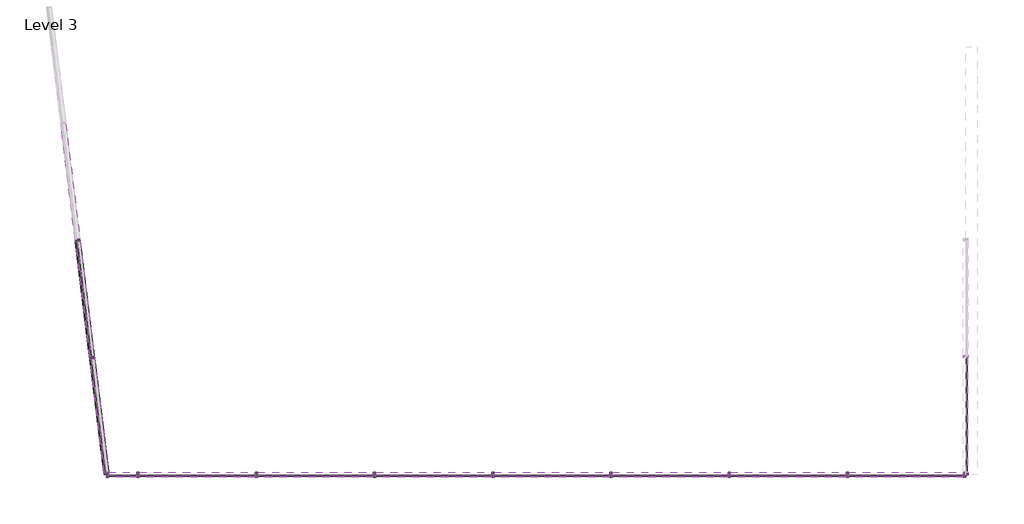
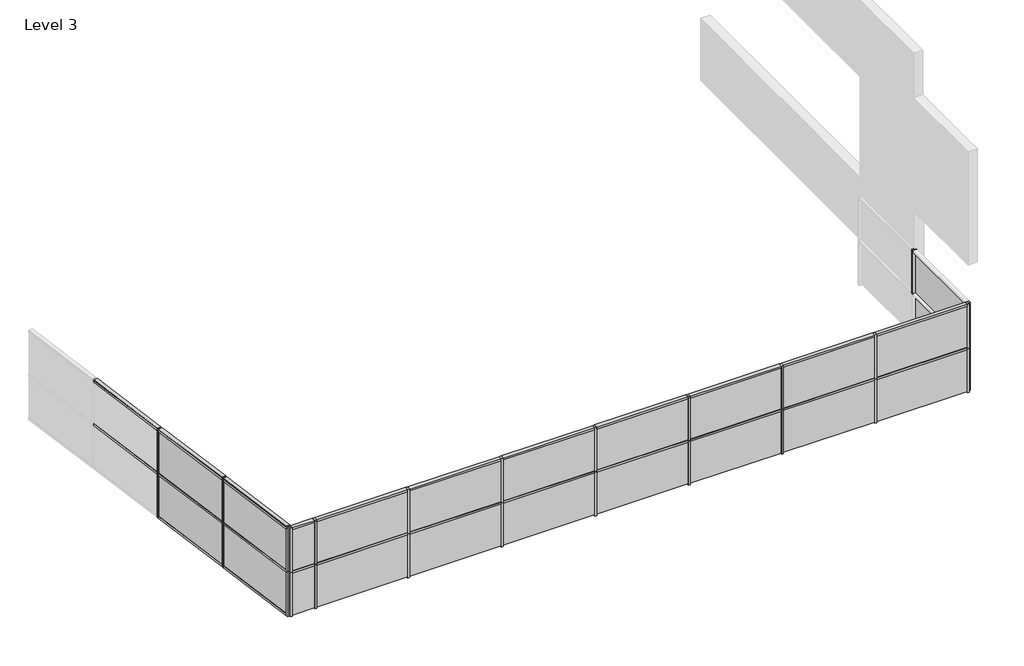
# One storey, part 1 of 2: 63 members, 26 plates.
"""IFC4 building model written with IfcOpenShell, lengths in millimetres."""

from ifc_helpers import new_model, si_unit, origin, place, context, project, spatial, transform, mapped, element, save
from components import member_71c27fd2, member_daa7a266, member_82905deb, member_19d0a4ec, member_8cef0660, member_db480205, member_4491d118, member_0c11e56c, member_695b83e4, system_panel_glazed_37f15d2e, system_panel_glazed_3620f98e, system_panel_glazed_e46d4b42, system_panel_glazed_2a6c68b7, system_panel_glazed_07b088f8, system_panel_glazed_9d0e0944

model = new_model("IFC4")

# Units and contexts
model_context = context("Model", 3, world=origin())
ifc_project = project(units=[si_unit("LENGTHUNIT", "METRE", prefix="MILLI")], contexts=[model_context])

# Site, building, storey
site = spatial("IfcSite", under=ifc_project)
building = spatial("IfcBuilding", under=site)
storey = spatial("IfcBuildingStorey", under=building, Name="Level 3", Elevation=6096.0)

# Members
placement = place(None, origin())
member_shape = member_71c27fd2(model_context)
element("IfcMember", 1, ObjectType="Rectangular Mullion : 2.5\" x 5\" rectangular", at=placement, inside=storey, context=model_context, shape_type="MappedRepresentation", body=[
    mapped(member_shape, transform((-8620.3262186, -3985.3690403, 6096.0), x_axis=(0.0, 0.0, -1.0), y_axis=(-0.9925461516413222, -0.12186934340514607, 0.0), z_axis=(-0.12186934340514607, 0.9925461516413222, 0.0))),
])
member_2_shape = member_daa7a266(model_context)
element("IfcMember", 2, ObjectType="Rectangular Mullion : 2.5\" x 5\" rectangular", at=placement, inside=storey, context=model_context, shape_type="MappedRepresentation", body=[
    mapped(member_2_shape, transform((-8260.4765148, -6916.1096898, 9144.0), x_axis=(0.0, 0.0, 1.0), y_axis=(-0.9925461516413222, -0.12186934340514603, 0.0), z_axis=(0.12186934340514603, -0.9925461516413222, 0.0))),
])
element("IfcMember", 3, ObjectType="Rectangular Mullion : 2.5\" x 5\" rectangular", at=placement, inside=storey, context=model_context, shape_type="MappedRepresentation", body=[
    mapped(member_2_shape, transform((13839.0156363, -6979.1363705, 9144.0), x_axis=(0.0, 0.0, 1.0), y_axis=(0.0, -1.0, 0.0), z_axis=(1.0, 0.0, 0.0))),
])
member_3_shape = member_82905deb(model_context)
element("IfcMember", 4, ObjectType="Rectangular Mullion : 2.5\" x 5\" rectangular", at=placement, inside=storey, context=model_context, shape_type="MappedRepresentation", body=[
    mapped(member_3_shape, transform((-8624.1955702, -3953.8557, 9144.0), x_axis=(-0.12186934340514591, 0.9925461516413222, 0.0), y_axis=(-0.9925461516413222, -0.12186934340514591, 0.0), z_axis=(0.0, 0.0, 1.0))),
])
element("IfcMember", 5, ObjectType="Rectangular Mullion : 2.5\" x 5\" rectangular", at=placement, inside=storey, context=model_context, shape_type="MappedRepresentation", body=[
    mapped(member_3_shape, transform((-8995.6533289, -928.5750297, 9144.0), x_axis=(-0.12186934340514591, 0.9925461516413222, 0.0), y_axis=(-0.9925461516413222, -0.12186934340514591, 0.0), z_axis=(0.0, 0.0, 1.0))),
])
element("IfcMember", 6, ObjectType="Rectangular Mullion : 2.5\" x 5\" rectangular", at=placement, inside=storey, context=model_context, shape_type="MappedRepresentation", body=[
    mapped(member_3_shape, transform((10854.515636, -6979.1363705, 9144.0), x_axis=(-1.0, 0.0, 0.0), y_axis=(0.0, -1.0, 0.0), z_axis=(0.0, 0.0, 1.0))),
])
element("IfcMember", 7, ObjectType="Rectangular Mullion : 2.5\" x 5\" rectangular", at=placement, inside=storey, context=model_context, shape_type="MappedRepresentation", body=[
    mapped(member_3_shape, transform((7806.515636, -6979.1363705, 9144.0), x_axis=(-1.0, 0.0, 0.0), y_axis=(0.0, -1.0, 0.0), z_axis=(0.0, 0.0, 1.0))),
])
element("IfcMember", 8, ObjectType="Rectangular Mullion : 2.5\" x 5\" rectangular", at=placement, inside=storey, context=model_context, shape_type="MappedRepresentation", body=[
    mapped(member_3_shape, transform((4758.515636, -6979.1363705, 9144.0), x_axis=(-1.0, 0.0, 0.0), y_axis=(0.0, -1.0, 0.0), z_axis=(0.0, 0.0, 1.0))),
])
element("IfcMember", 9, ObjectType="Rectangular Mullion : 2.5\" x 5\" rectangular", at=placement, inside=storey, context=model_context, shape_type="MappedRepresentation", body=[
    mapped(member_3_shape, transform((1710.515636, -6979.1363705, 9144.0), x_axis=(-1.0, 0.0, 0.0), y_axis=(0.0, -1.0, 0.0), z_axis=(0.0, 0.0, 1.0))),
])
element("IfcMember", 10, ObjectType="Rectangular Mullion : 2.5\" x 5\" rectangular", at=placement, inside=storey, context=model_context, shape_type="MappedRepresentation", body=[
    mapped(member_3_shape, transform((-1337.484364, -6979.1363705, 9144.0), x_axis=(-1.0, 0.0, 0.0), y_axis=(0.0, -1.0, 0.0), z_axis=(0.0, 0.0, 1.0))),
])
element("IfcMember", 11, ObjectType="Rectangular Mullion : 2.5\" x 5\" rectangular", at=placement, inside=storey, context=model_context, shape_type="MappedRepresentation", body=[
    mapped(member_3_shape, transform((-4385.484364, -6979.1363705, 9144.0), x_axis=(-1.0, 0.0, 0.0), y_axis=(0.0, -1.0, 0.0), z_axis=(0.0, 0.0, 1.0))),
])
element("IfcMember", 12, ObjectType="Rectangular Mullion : 2.5\" x 5\" rectangular", at=placement, inside=storey, context=model_context, shape_type="MappedRepresentation", body=[
    mapped(member_3_shape, transform((-7433.484364, -6979.1363705, 9144.0), x_axis=(-1.0, 0.0, 0.0), y_axis=(0.0, -1.0, 0.0), z_axis=(0.0, 0.0, 1.0))),
])
element("IfcMember", 13, ObjectType="Rectangular Mullion : 2.5\" x 5\" rectangular", at=placement, inside=storey, context=model_context, shape_type="MappedRepresentation", body=[
    mapped(member_3_shape, transform((13902.5156363, -3931.1363708, 9144.0), x_axis=(0.0, -1.0, 0.0), y_axis=(1.0, 0.0, 0.0), z_axis=(0.0, 0.0, 1.0))),
])
member_4_shape = member_19d0a4ec(model_context)
element("IfcMember", 14, ObjectType="Rectangular Mullion : 2.5\" x 5\" rectangular", at=placement, inside=storey, context=model_context, shape_type="MappedRepresentation", body=[
    mapped(member_4_shape, transform((-8260.4765148, -6916.1096898, 7620.0), x_axis=(0.0, 0.0, 1.0), y_axis=(-0.9925461516413222, -0.12186934340514587, 0.0), z_axis=(0.12186934340514587, -0.9925461516413222, 0.0))),
])
element("IfcMember", 15, ObjectType="Rectangular Mullion : 2.5\" x 5\" rectangular", at=placement, inside=storey, context=model_context, shape_type="MappedRepresentation", body=[
    mapped(member_4_shape, transform((13839.0156363, -6979.1363705, 7620.0), x_axis=(0.0, 0.0, 1.0), y_axis=(0.0, -1.0, 0.0), z_axis=(1.0, 0.0, 0.0))),
])
element("IfcMember", 16, ObjectType="Rectangular Mullion : 2.5\" x 5\" rectangular", at=placement, inside=storey, context=model_context, shape_type="MappedRepresentation", body=[
    mapped(member_4_shape, transform((-8260.4765148, -6916.1096898, 7620.0), x_axis=(0.0, 0.0, 1.0), y_axis=(-0.9925461516413222, -0.12186934340514591, 0.0), z_axis=(0.12186934340514591, -0.9925461516413222, 0.0))),
])
element("IfcMember", 17, ObjectType="Rectangular Mullion : 2.5\" x 5\" rectangular", at=placement, inside=storey, context=model_context, shape_type="MappedRepresentation", body=[
    mapped(member_4_shape, transform((-8260.4765148, -6916.1096898, 9144.0), x_axis=(0.0, 0.0, 1.0), y_axis=(-0.9925461516413223, -0.12186934340514574, 0.0), z_axis=(0.12186934340514574, -0.9925461516413223, 0.0))),
])
member_5_shape = member_8cef0660(model_context)
element("IfcMember", 18, ObjectType="Rectangular Mullion : 2.5\" x 5\" rectangular", at=placement, inside=storey, context=model_context, shape_type="MappedRepresentation", body=[
    mapped(member_5_shape, transform((-8628.0649219, -3922.3423596, 7620.0), x_axis=(0.0, 0.0, 1.0), y_axis=(-0.9925461516413222, -0.12186934340514596, 0.0), z_axis=(0.12186934340514596, -0.9925461516413222, 0.0))),
])
element("IfcMember", 19, ObjectType="Rectangular Mullion : 2.5\" x 5\" rectangular", at=placement, inside=storey, context=model_context, shape_type="MappedRepresentation", body=[
    mapped(member_5_shape, transform((-8999.5226806, -897.0616894, 7620.0), x_axis=(0.0, 0.0, 1.0), y_axis=(-0.9925461516413222, -0.12186934340514602, 0.0), z_axis=(0.12186934340514602, -0.9925461516413222, 0.0))),
])
element("IfcMember", 20, ObjectType="Rectangular Mullion : 2.5\" x 5\" rectangular", at=placement, inside=storey, context=model_context, shape_type="MappedRepresentation", body=[
    mapped(member_5_shape, transform((10822.765636, -6979.1363705, 7620.0), x_axis=(0.0, 0.0, 1.0), y_axis=(0.0, -1.0, 0.0), z_axis=(1.0, 0.0, 0.0))),
])
element("IfcMember", 21, ObjectType="Rectangular Mullion : 2.5\" x 5\" rectangular", at=placement, inside=storey, context=model_context, shape_type="MappedRepresentation", body=[
    mapped(member_5_shape, transform((7774.765636, -6979.1363705, 7620.0), x_axis=(0.0, 0.0, 1.0), y_axis=(0.0, -1.0, 0.0), z_axis=(1.0, 0.0, 0.0))),
])
element("IfcMember", 22, ObjectType="Rectangular Mullion : 2.5\" x 5\" rectangular", at=placement, inside=storey, context=model_context, shape_type="MappedRepresentation", body=[
    mapped(member_5_shape, transform((4726.765636, -6979.1363705, 7620.0), x_axis=(0.0, 0.0, 1.0), y_axis=(0.0, -1.0, 0.0), z_axis=(1.0, 0.0, 0.0))),
])
element("IfcMember", 23, ObjectType="Rectangular Mullion : 2.5\" x 5\" rectangular", at=placement, inside=storey, context=model_context, shape_type="MappedRepresentation", body=[
    mapped(member_5_shape, transform((1678.765636, -6979.1363705, 7620.0), x_axis=(0.0, 0.0, 1.0), y_axis=(0.0, -1.0, 0.0), z_axis=(1.0, 0.0, 0.0))),
])
element("IfcMember", 24, ObjectType="Rectangular Mullion : 2.5\" x 5\" rectangular", at=placement, inside=storey, context=model_context, shape_type="MappedRepresentation", body=[
    mapped(member_5_shape, transform((-1369.234364, -6979.1363705, 7620.0), x_axis=(0.0, 0.0, 1.0), y_axis=(0.0, -1.0, 0.0), z_axis=(1.0, 0.0, 0.0))),
])
element("IfcMember", 25, ObjectType="Rectangular Mullion : 2.5\" x 5\" rectangular", at=placement, inside=storey, context=model_context, shape_type="MappedRepresentation", body=[
    mapped(member_5_shape, transform((-4417.234364, -6979.1363705, 7620.0), x_axis=(0.0, 0.0, 1.0), y_axis=(0.0, -1.0, 0.0), z_axis=(1.0, 0.0, 0.0))),
])
element("IfcMember", 26, ObjectType="Rectangular Mullion : 2.5\" x 5\" rectangular", at=placement, inside=storey, context=model_context, shape_type="MappedRepresentation", body=[
    mapped(member_5_shape, transform((-8628.0649219, -3922.3423596, 7620.0), x_axis=(0.0, 0.0, 1.0), y_axis=(-0.9925461516413222, -0.12186934340514592, 0.0), z_axis=(0.12186934340514592, -0.9925461516413222, 0.0))),
])
element("IfcMember", 27, ObjectType="Rectangular Mullion : 2.5\" x 5\" rectangular", at=placement, inside=storey, context=model_context, shape_type="MappedRepresentation", body=[
    mapped(member_5_shape, transform((-8999.5226806, -897.0616894, 7620.0), x_axis=(0.0, 0.0, 1.0), y_axis=(-0.9925461516413222, -0.12186934340514566, 0.0), z_axis=(0.12186934340514566, -0.9925461516413222, 0.0))),
])
element("IfcMember", 28, ObjectType="Rectangular Mullion : 2.5\" x 5\" rectangular", at=placement, inside=storey, context=model_context, shape_type="MappedRepresentation", body=[
    mapped(member_5_shape, transform((-8628.0649219, -3922.3423596, 9144.0), x_axis=(0.0, 0.0, 1.0), y_axis=(-0.9925461516413222, -0.12186934340514592, 0.0), z_axis=(0.12186934340514592, -0.9925461516413222, 0.0))),
])
element("IfcMember", 29, ObjectType="Rectangular Mullion : 2.5\" x 5\" rectangular", at=placement, inside=storey, context=model_context, shape_type="MappedRepresentation", body=[
    mapped(member_5_shape, transform((-8999.5226806, -897.0616894, 9144.0), x_axis=(0.0, 0.0, 1.0), y_axis=(-0.9925461516413222, -0.12186934340514602, 0.0), z_axis=(0.12186934340514602, -0.9925461516413222, 0.0))),
])
member_6_shape = member_db480205(model_context)
element("IfcMember", 30, ObjectType="Rectangular Mullion : 2.5\" x 5\" rectangular", at=placement, inside=storey, context=model_context, shape_type="MappedRepresentation", body=[
    mapped(member_6_shape, transform((-8991.7839773, -960.0883701, 6096.0), x_axis=(0.0, 0.0, -1.0), y_axis=(-0.9925461516413222, -0.12186934340514592, 0.0), z_axis=(-0.12186934340514592, 0.9925461516413222, 0.0))),
])
element("IfcMember", 31, ObjectType="Rectangular Mullion : 2.5\" x 5\" rectangular", at=placement, inside=storey, context=model_context, shape_type="MappedRepresentation", body=[
    mapped(member_6_shape, transform((-8628.0649219, -3922.3423596, 9144.0), x_axis=(0.0, 0.0, 1.0), y_axis=(-0.9925461516413222, -0.12186934340514595, 0.0), z_axis=(0.12186934340514595, -0.9925461516413222, 0.0))),
])
element("IfcMember", 32, ObjectType="Rectangular Mullion : 2.5\" x 5\" rectangular", at=placement, inside=storey, context=model_context, shape_type="MappedRepresentation", body=[
    mapped(member_6_shape, transform((-8999.5226806, -897.0616894, 9144.0), x_axis=(0.0, 0.0, 1.0), y_axis=(-0.9925461516413222, -0.12186934340514596, 0.0), z_axis=(0.12186934340514596, -0.9925461516413222, 0.0))),
])
element("IfcMember", 33, ObjectType="Rectangular Mullion : 2.5\" x 5\" rectangular", at=placement, inside=storey, context=model_context, shape_type="MappedRepresentation", body=[
    mapped(member_6_shape, transform((10822.765636, -6979.1363705, 9144.0), x_axis=(0.0, 0.0, 1.0), y_axis=(0.0, -1.0, 0.0), z_axis=(1.0, 0.0, 0.0))),
])
element("IfcMember", 34, ObjectType="Rectangular Mullion : 2.5\" x 5\" rectangular", at=placement, inside=storey, context=model_context, shape_type="MappedRepresentation", body=[
    mapped(member_6_shape, transform((7774.765636, -6979.1363705, 9144.0), x_axis=(0.0, 0.0, 1.0), y_axis=(0.0, -1.0, 0.0), z_axis=(1.0, 0.0, 0.0))),
])
element("IfcMember", 35, ObjectType="Rectangular Mullion : 2.5\" x 5\" rectangular", at=placement, inside=storey, context=model_context, shape_type="MappedRepresentation", body=[
    mapped(member_6_shape, transform((4726.765636, -6979.1363705, 9144.0), x_axis=(0.0, 0.0, 1.0), y_axis=(0.0, -1.0, 0.0), z_axis=(1.0, 0.0, 0.0))),
])
element("IfcMember", 36, ObjectType="Rectangular Mullion : 2.5\" x 5\" rectangular", at=placement, inside=storey, context=model_context, shape_type="MappedRepresentation", body=[
    mapped(member_6_shape, transform((1678.765636, -6979.1363705, 9144.0), x_axis=(0.0, 0.0, 1.0), y_axis=(0.0, -1.0, 0.0), z_axis=(1.0, 0.0, 0.0))),
])
element("IfcMember", 37, ObjectType="Rectangular Mullion : 2.5\" x 5\" rectangular", at=placement, inside=storey, context=model_context, shape_type="MappedRepresentation", body=[
    mapped(member_6_shape, transform((-1369.234364, -6979.1363705, 9144.0), x_axis=(0.0, 0.0, 1.0), y_axis=(0.0, -1.0, 0.0), z_axis=(1.0, 0.0, 0.0))),
])
element("IfcMember", 38, ObjectType="Rectangular Mullion : 2.5\" x 5\" rectangular", at=placement, inside=storey, context=model_context, shape_type="MappedRepresentation", body=[
    mapped(member_6_shape, transform((-4417.234364, -6979.1363705, 9144.0), x_axis=(0.0, 0.0, 1.0), y_axis=(0.0, -1.0, 0.0), z_axis=(1.0, 0.0, 0.0))),
])
element("IfcMember", 39, ObjectType="Rectangular Mullion : 2.5\" x 5\" rectangular", at=placement, inside=storey, context=model_context, shape_type="MappedRepresentation", body=[
    mapped(member_3_shape, transform((-8624.1955702, -3953.8557, 7620.0), x_axis=(-0.1218693434051459, 0.9925461516413222, 0.0), y_axis=(-0.9925461516413222, -0.1218693434051459, 0.0), z_axis=(0.0, 0.0, 1.0))),
])
element("IfcMember", 40, ObjectType="Rectangular Mullion : 2.5\" x 5\" rectangular", at=placement, inside=storey, context=model_context, shape_type="MappedRepresentation", body=[
    mapped(member_3_shape, transform((-8995.6533289, -928.5750297, 7620.0), x_axis=(-0.1218693434051459, 0.9925461516413222, 0.0), y_axis=(-0.9925461516413222, -0.1218693434051459, 0.0), z_axis=(0.0, 0.0, 1.0))),
])
element("IfcMember", 41, ObjectType="Rectangular Mullion : 2.5\" x 5\" rectangular", at=placement, inside=storey, context=model_context, shape_type="MappedRepresentation", body=[
    mapped(member_3_shape, transform((-8624.1955702, -3953.8557, 7620.0), x_axis=(-0.12186934340514591, 0.9925461516413222, 0.0), y_axis=(-0.9925461516413222, -0.12186934340514591, 0.0), z_axis=(0.0, 0.0, 1.0))),
])
element("IfcMember", 42, ObjectType="Rectangular Mullion : 2.5\" x 5\" rectangular", at=placement, inside=storey, context=model_context, shape_type="MappedRepresentation", body=[
    mapped(member_3_shape, transform((-8995.6533289, -928.5750297, 7620.0), x_axis=(-0.12186934340514591, 0.9925461516413222, 0.0), y_axis=(-0.9925461516413222, -0.12186934340514591, 0.0), z_axis=(0.0, 0.0, 1.0))),
])
element("IfcMember", 43, ObjectType="Rectangular Mullion : 2.5\" x 5\" rectangular", at=placement, inside=storey, context=model_context, shape_type="MappedRepresentation", body=[
    mapped(member_3_shape, transform((10854.515636, -6979.1363705, 7620.0), x_axis=(-1.0, 0.0, 0.0), y_axis=(0.0, -1.0, 0.0), z_axis=(0.0, 0.0, 1.0))),
])
element("IfcMember", 44, ObjectType="Rectangular Mullion : 2.5\" x 5\" rectangular", at=placement, inside=storey, context=model_context, shape_type="MappedRepresentation", body=[
    mapped(member_3_shape, transform((7806.515636, -6979.1363705, 7620.0), x_axis=(-1.0, 0.0, 0.0), y_axis=(0.0, -1.0, 0.0), z_axis=(0.0, 0.0, 1.0))),
])
element("IfcMember", 45, ObjectType="Rectangular Mullion : 2.5\" x 5\" rectangular", at=placement, inside=storey, context=model_context, shape_type="MappedRepresentation", body=[
    mapped(member_3_shape, transform((4758.515636, -6979.1363705, 7620.0), x_axis=(-1.0, 0.0, 0.0), y_axis=(0.0, -1.0, 0.0), z_axis=(0.0, 0.0, 1.0))),
])
element("IfcMember", 46, ObjectType="Rectangular Mullion : 2.5\" x 5\" rectangular", at=placement, inside=storey, context=model_context, shape_type="MappedRepresentation", body=[
    mapped(member_3_shape, transform((1710.515636, -6979.1363705, 7620.0), x_axis=(-1.0, 0.0, 0.0), y_axis=(0.0, -1.0, 0.0), z_axis=(0.0, 0.0, 1.0))),
])
element("IfcMember", 47, ObjectType="Rectangular Mullion : 2.5\" x 5\" rectangular", at=placement, inside=storey, context=model_context, shape_type="MappedRepresentation", body=[
    mapped(member_3_shape, transform((-1337.484364, -6979.1363705, 7620.0), x_axis=(-1.0, 0.0, 0.0), y_axis=(0.0, -1.0, 0.0), z_axis=(0.0, 0.0, 1.0))),
])
element("IfcMember", 48, ObjectType="Rectangular Mullion : 2.5\" x 5\" rectangular", at=placement, inside=storey, context=model_context, shape_type="MappedRepresentation", body=[
    mapped(member_3_shape, transform((-4385.484364, -6979.1363705, 7620.0), x_axis=(-1.0, 0.0, 0.0), y_axis=(0.0, -1.0, 0.0), z_axis=(0.0, 0.0, 1.0))),
])
element("IfcMember", 49, ObjectType="Rectangular Mullion : 2.5\" x 5\" rectangular", at=placement, inside=storey, context=model_context, shape_type="MappedRepresentation", body=[
    mapped(member_3_shape, transform((-7433.484364, -6979.1363705, 7620.0), x_axis=(-1.0, 0.0, 0.0), y_axis=(0.0, -1.0, 0.0), z_axis=(0.0, 0.0, 1.0))),
])
element("IfcMember", 50, ObjectType="Rectangular Mullion : 2.5\" x 5\" rectangular", at=placement, inside=storey, context=model_context, shape_type="MappedRepresentation", body=[
    mapped(member_3_shape, transform((-8624.1955702, -3953.8557, 9144.0), x_axis=(-0.1218693434051459, 0.9925461516413222, 0.0), y_axis=(-0.9925461516413222, -0.1218693434051459, 0.0), z_axis=(0.0, 0.0, 1.0))),
])
element("IfcMember", 51, ObjectType="Rectangular Mullion : 2.5\" x 5\" rectangular", at=placement, inside=storey, context=model_context, shape_type="MappedRepresentation", body=[
    mapped(member_3_shape, transform((-8995.6533289, -928.5750297, 9144.0), x_axis=(-0.1218693434051459, 0.9925461516413222, 0.0), y_axis=(-0.9925461516413222, -0.1218693434051459, 0.0), z_axis=(0.0, 0.0, 1.0))),
])
member_7_shape = member_4491d118(model_context)
element("IfcMember", 52, ObjectType="Rectangular Mullion : 2.5\" x 5\" rectangular", at=placement, inside=storey, context=model_context, shape_type="MappedRepresentation", body=[
    mapped(member_7_shape, transform((-8252.7378115, -6979.1363705, 9144.0), x_axis=(-1.0, 0.0, 0.0), y_axis=(0.0, -1.0, 0.0), z_axis=(0.0, 0.0, 1.0))),
])
element("IfcMember", 53, ObjectType="Rectangular Mullion : 2.5\" x 5\" rectangular", at=placement, inside=storey, context=model_context, shape_type="MappedRepresentation", body=[
    mapped(member_7_shape, transform((13902.5156363, -6979.1363705, 9144.0), x_axis=(0.0, -1.0, 0.0), y_axis=(1.0, 0.0, 0.0), z_axis=(0.0, 0.0, 1.0))),
])
element("IfcMember", 54, ObjectType="Rectangular Mullion : 2.5\" x 5\" rectangular", at=placement, inside=storey, context=model_context, shape_type="MappedRepresentation", body=[
    mapped(member_7_shape, transform((-8252.7378115, -6979.1363705, 6096.0), x_axis=(0.1218693434051459, -0.9925461516413222, 0.0), y_axis=(-0.9925461516413222, -0.1218693434051459, 0.0), z_axis=(0.0, 0.0, -1.0))),
])
element("IfcMember", 55, ObjectType="Rectangular Mullion : 2.5\" x 5\" rectangular", at=placement, inside=storey, context=model_context, shape_type="MappedRepresentation", body=[
    mapped(member_7_shape, transform((-8252.7378115, -6979.1363705, 6096.0), x_axis=(0.12186934340514591, -0.9925461516413222, 0.0), y_axis=(-0.9925461516413222, -0.12186934340514591, 0.0), z_axis=(0.0, 0.0, -1.0))),
])
element("IfcMember", 56, ObjectType="Rectangular Mullion : 2.5\" x 5\" rectangular", at=placement, inside=storey, context=model_context, shape_type="MappedRepresentation", body=[
    mapped(member_7_shape, transform((13902.5156363, -6979.1363705, 6096.0), x_axis=(1.0, 0.0, 0.0), y_axis=(0.0, -1.0, 0.0), z_axis=(0.0, 0.0, -1.0))),
])
element("IfcMember", 57, ObjectType="Rectangular Mullion : 2.5\" x 5\" rectangular", at=placement, inside=storey, context=model_context, shape_type="MappedRepresentation", body=[
    mapped(member_7_shape, transform((-8252.7378115, -6979.1363705, 7620.0), x_axis=(0.1218693434051459, -0.9925461516413222, 0.0), y_axis=(-0.9925461516413222, -0.1218693434051459, 0.0), z_axis=(0.0, 0.0, -1.0))),
])
element("IfcMember", 58, ObjectType="Rectangular Mullion : 2.5\" x 5\" rectangular", at=placement, inside=storey, context=model_context, shape_type="MappedRepresentation", body=[
    mapped(member_7_shape, transform((-8252.7378115, -6979.1363705, 7620.0), x_axis=(0.12186934340514591, -0.9925461516413222, 0.0), y_axis=(-0.9925461516413222, -0.12186934340514591, 0.0), z_axis=(0.0, 0.0, -1.0))),
])
element("IfcMember", 59, ObjectType="Rectangular Mullion : 2.5\" x 5\" rectangular", at=placement, inside=storey, context=model_context, shape_type="MappedRepresentation", body=[
    mapped(member_7_shape, transform((13902.5156363, -6979.1363705, 7620.0), x_axis=(1.0, 0.0, 0.0), y_axis=(0.0, -1.0, 0.0), z_axis=(0.0, 0.0, -1.0))),
])
element("IfcMember", 60, ObjectType="Rectangular Mullion : 2.5\" x 5\" rectangular", at=placement, inside=storey, context=model_context, shape_type="MappedRepresentation", body=[
    mapped(member_7_shape, transform((-8252.7378115, -6979.1363705, 7620.0), x_axis=(-1.0, 0.0, 0.0), y_axis=(0.0, -1.0, 0.0), z_axis=(0.0, 0.0, 1.0))),
])
element("IfcMember", 61, ObjectType="Rectangular Mullion : 2.5\" x 5\" rectangular", at=placement, inside=storey, context=model_context, shape_type="MappedRepresentation", body=[
    mapped(member_7_shape, transform((13902.5156363, -6979.1363705, 7620.0), x_axis=(0.0, -1.0, 0.0), y_axis=(1.0, 0.0, 0.0), z_axis=(0.0, 0.0, 1.0))),
])
member_8_shape = member_0c11e56c(model_context)
element("IfcMember", 62, ObjectType="Rectangular Mullion : 2.5\" x 5\" rectangular", at=placement, inside=storey, context=model_context, shape_type="MappedRepresentation", body=[
    mapped(member_8_shape, transform((-7465.234364, -6979.1363705, 7620.0), x_axis=(0.0, 0.0, 1.0), y_axis=(0.0, -1.0, 0.0), z_axis=(1.0, 0.0, 0.0))),
])
member_9_shape = member_695b83e4(model_context)
element("IfcMember", 63, ObjectType="Rectangular Mullion : 2.5\" x 5\" rectangular", at=placement, inside=storey, context=model_context, shape_type="MappedRepresentation", body=[
    mapped(member_9_shape, transform((-7465.234364, -6979.1363705, 9144.0), x_axis=(0.0, 0.0, 1.0), y_axis=(0.0, -1.0, 0.0), z_axis=(1.0, 0.0, 0.0))),
])

# Plates
system_panel_glazed_shape = system_panel_glazed_37f15d2e(model_context)
element("IfcPlate", 64, ObjectType="System Panel : Glazed", at=placement, inside=storey, context=model_context, shape_type="MappedRepresentation", body=[
    mapped(system_panel_glazed_shape, transform((-8440.4013667, -5450.739365, 6159.5), x_axis=(-0.1218693434051459, 0.9925461516413222, 0.0), y_axis=(-0.9925461516413222, -0.1218693434051459, 0.0), z_axis=(0.0, 0.0, 1.0))),
])
element("IfcPlate", 65, ObjectType="System Panel : Glazed", at=placement, inside=storey, context=model_context, shape_type="MappedRepresentation", body=[
    mapped(system_panel_glazed_shape, transform((-8440.4013667, -5450.739365, 7651.75), x_axis=(-0.12186934340514591, 0.9925461516413222, 0.0), y_axis=(-0.9925461516413222, -0.12186934340514591, 0.0), z_axis=(0.0, 0.0, 1.0))),
])
element("IfcPlate", 66, ObjectType="System Panel : Glazed", at=placement, inside=storey, context=model_context, shape_type="MappedRepresentation", body=[
    mapped(system_panel_glazed_shape, transform((12362.6406361, -6979.1363705, 7651.75), x_axis=(-1.0, 0.0, 0.0), y_axis=(0.0, -1.0, 0.0), z_axis=(0.0, 0.0, 1.0))),
])
element("IfcPlate", 67, ObjectType="System Panel : Glazed", at=placement, inside=storey, context=model_context, shape_type="MappedRepresentation", body=[
    mapped(system_panel_glazed_shape, transform((13902.5156363, -5439.2613706, 7651.75), x_axis=(0.0, -1.0, 0.0), y_axis=(1.0, 0.0, 0.0), z_axis=(0.0, 0.0, 1.0))),
])
system_panel_glazed_2_shape = system_panel_glazed_3620f98e(model_context)
element("IfcPlate", 68, ObjectType="System Panel : Glazed", at=placement, inside=storey, context=model_context, shape_type="MappedRepresentation", body=[
    mapped(system_panel_glazed_2_shape, transform((-8809.9244496, -2441.2153649, 7651.75), x_axis=(-0.12186934340514591, 0.9925461516413222, 0.0), y_axis=(-0.9925461516413222, -0.12186934340514591, 0.0), z_axis=(0.0, 0.0, 1.0))),
])
element("IfcPlate", 69, ObjectType="System Panel : Glazed", at=placement, inside=storey, context=model_context, shape_type="MappedRepresentation", body=[
    mapped(system_panel_glazed_2_shape, transform((9330.515636, -6979.1363705, 7651.75), x_axis=(-1.0, 0.0, 0.0), y_axis=(0.0, -1.0, 0.0), z_axis=(0.0, 0.0, 1.0))),
])
element("IfcPlate", 70, ObjectType="System Panel : Glazed", at=placement, inside=storey, context=model_context, shape_type="MappedRepresentation", body=[
    mapped(system_panel_glazed_2_shape, transform((6282.515636, -6979.1363705, 7651.75), x_axis=(-1.0, 0.0, 0.0), y_axis=(0.0, -1.0, 0.0), z_axis=(0.0, 0.0, 1.0))),
])
element("IfcPlate", 71, ObjectType="System Panel : Glazed", at=placement, inside=storey, context=model_context, shape_type="MappedRepresentation", body=[
    mapped(system_panel_glazed_2_shape, transform((3234.515636, -6979.1363705, 7651.75), x_axis=(-1.0, 0.0, 0.0), y_axis=(0.0, -1.0, 0.0), z_axis=(0.0, 0.0, 1.0))),
])
element("IfcPlate", 72, ObjectType="System Panel : Glazed", at=placement, inside=storey, context=model_context, shape_type="MappedRepresentation", body=[
    mapped(system_panel_glazed_2_shape, transform((186.515636, -6979.1363705, 7651.75), x_axis=(-1.0, 0.0, 0.0), y_axis=(0.0, -1.0, 0.0), z_axis=(0.0, 0.0, 1.0))),
])
element("IfcPlate", 73, ObjectType="System Panel : Glazed", at=placement, inside=storey, context=model_context, shape_type="MappedRepresentation", body=[
    mapped(system_panel_glazed_2_shape, transform((-2861.484364, -6979.1363705, 7651.75), x_axis=(-1.0, 0.0, 0.0), y_axis=(0.0, -1.0, 0.0), z_axis=(0.0, 0.0, 1.0))),
])
element("IfcPlate", 74, ObjectType="System Panel : Glazed", at=placement, inside=storey, context=model_context, shape_type="MappedRepresentation", body=[
    mapped(system_panel_glazed_2_shape, transform((-5909.484364, -6979.1363705, 7651.75), x_axis=(-1.0, 0.0, 0.0), y_axis=(0.0, -1.0, 0.0), z_axis=(0.0, 0.0, 1.0))),
])
element("IfcPlate", 75, ObjectType="System Panel : Glazed", at=placement, inside=storey, context=model_context, shape_type="MappedRepresentation", body=[
    mapped(system_panel_glazed_2_shape, transform((-8809.9244496, -2441.2153649, 6159.5), x_axis=(-0.1218693434051459, 0.9925461516413222, 0.0), y_axis=(-0.9925461516413222, -0.1218693434051459, 0.0), z_axis=(0.0, 0.0, 1.0))),
])
system_panel_glazed_3_shape = system_panel_glazed_e46d4b42(model_context)
element("IfcPlate", 76, ObjectType="System Panel : Glazed", at=placement, inside=storey, context=model_context, shape_type="MappedRepresentation", body=[
    mapped(system_panel_glazed_3_shape, transform((-8440.4013667, -5450.739365, 6127.75), x_axis=(-0.12186934340514591, 0.9925461516413222, 0.0), y_axis=(-0.9925461516413222, -0.12186934340514591, 0.0), z_axis=(0.0, 0.0, 1.0))),
])
element("IfcPlate", 77, ObjectType="System Panel : Glazed", at=placement, inside=storey, context=model_context, shape_type="MappedRepresentation", body=[
    mapped(system_panel_glazed_3_shape, transform((12362.6406361, -6979.1363705, 6127.75), x_axis=(-1.0, 0.0, 0.0), y_axis=(0.0, -1.0, 0.0), z_axis=(0.0, 0.0, 1.0))),
])
element("IfcPlate", 78, ObjectType="System Panel : Glazed", at=placement, inside=storey, context=model_context, shape_type="MappedRepresentation", body=[
    mapped(system_panel_glazed_3_shape, transform((13902.5156363, -5439.2613706, 6127.75), x_axis=(0.0, -1.0, 0.0), y_axis=(1.0, 0.0, 0.0), z_axis=(0.0, 0.0, 1.0))),
])
element("IfcPlate", 79, ObjectType="System Panel : Glazed", at=placement, inside=storey, context=model_context, shape_type="MappedRepresentation", body=[
    mapped(system_panel_glazed_3_shape, transform((-8440.4013667, -5450.739365, 7651.75), x_axis=(-0.1218693434051459, 0.9925461516413222, 0.0), y_axis=(-0.9925461516413222, -0.1218693434051459, 0.0), z_axis=(0.0, 0.0, 1.0))),
])
system_panel_glazed_4_shape = system_panel_glazed_2a6c68b7(model_context)
element("IfcPlate", 80, ObjectType="System Panel : Glazed", at=placement, inside=storey, context=model_context, shape_type="MappedRepresentation", body=[
    mapped(system_panel_glazed_4_shape, transform((-8809.9244496, -2441.2153649, 6127.75), x_axis=(-0.12186934340514591, 0.9925461516413222, 0.0), y_axis=(-0.9925461516413222, -0.12186934340514591, 0.0), z_axis=(0.0, 0.0, 1.0))),
])
element("IfcPlate", 81, ObjectType="System Panel : Glazed", at=placement, inside=storey, context=model_context, shape_type="MappedRepresentation", body=[
    mapped(system_panel_glazed_4_shape, transform((9330.515636, -6979.1363705, 6127.75), x_axis=(-1.0, 0.0, 0.0), y_axis=(0.0, -1.0, 0.0), z_axis=(0.0, 0.0, 1.0))),
])
element("IfcPlate", 82, ObjectType="System Panel : Glazed", at=placement, inside=storey, context=model_context, shape_type="MappedRepresentation", body=[
    mapped(system_panel_glazed_4_shape, transform((6282.515636, -6979.1363705, 6127.75), x_axis=(-1.0, 0.0, 0.0), y_axis=(0.0, -1.0, 0.0), z_axis=(0.0, 0.0, 1.0))),
])
element("IfcPlate", 83, ObjectType="System Panel : Glazed", at=placement, inside=storey, context=model_context, shape_type="MappedRepresentation", body=[
    mapped(system_panel_glazed_4_shape, transform((3234.515636, -6979.1363705, 6127.75), x_axis=(-1.0, 0.0, 0.0), y_axis=(0.0, -1.0, 0.0), z_axis=(0.0, 0.0, 1.0))),
])
element("IfcPlate", 84, ObjectType="System Panel : Glazed", at=placement, inside=storey, context=model_context, shape_type="MappedRepresentation", body=[
    mapped(system_panel_glazed_4_shape, transform((186.515636, -6979.1363705, 6127.75), x_axis=(-1.0, 0.0, 0.0), y_axis=(0.0, -1.0, 0.0), z_axis=(0.0, 0.0, 1.0))),
])
element("IfcPlate", 85, ObjectType="System Panel : Glazed", at=placement, inside=storey, context=model_context, shape_type="MappedRepresentation", body=[
    mapped(system_panel_glazed_4_shape, transform((-2861.484364, -6979.1363705, 6127.75), x_axis=(-1.0, 0.0, 0.0), y_axis=(0.0, -1.0, 0.0), z_axis=(0.0, 0.0, 1.0))),
])
element("IfcPlate", 86, ObjectType="System Panel : Glazed", at=placement, inside=storey, context=model_context, shape_type="MappedRepresentation", body=[
    mapped(system_panel_glazed_4_shape, transform((-5909.484364, -6979.1363705, 6127.75), x_axis=(-1.0, 0.0, 0.0), y_axis=(0.0, -1.0, 0.0), z_axis=(0.0, 0.0, 1.0))),
])
element("IfcPlate", 87, ObjectType="System Panel : Glazed", at=placement, inside=storey, context=model_context, shape_type="MappedRepresentation", body=[
    mapped(system_panel_glazed_4_shape, transform((-8809.9244496, -2441.2153649, 7651.75), x_axis=(-0.1218693434051459, 0.9925461516413222, 0.0), y_axis=(-0.9925461516413222, -0.1218693434051459, 0.0), z_axis=(0.0, 0.0, 1.0))),
])
system_panel_glazed_5_shape = system_panel_glazed_07b088f8(model_context)
element("IfcPlate", 88, ObjectType="System Panel : Glazed", at=placement, inside=storey, context=model_context, shape_type="MappedRepresentation", body=[
    mapped(system_panel_glazed_5_shape, transform((-7827.2360878, -6979.1363705, 7651.75), x_axis=(-1.0, 0.0, 0.0), y_axis=(0.0, -1.0, 0.0), z_axis=(0.0, 0.0, 1.0))),
])
system_panel_glazed_6_shape = system_panel_glazed_9d0e0944(model_context)
element("IfcPlate", 89, ObjectType="System Panel : Glazed", at=placement, inside=storey, context=model_context, shape_type="MappedRepresentation", body=[
    mapped(system_panel_glazed_6_shape, transform((-7827.2360878, -6979.1363705, 6127.75), x_axis=(-1.0, 0.0, 0.0), y_axis=(0.0, -1.0, 0.0), z_axis=(0.0, 0.0, 1.0))),
])

save(model, "model.ifc")

# Revit data of these elements
# Type "Rectangular Mullion : 2.5\" x 5\" rectangular"
#   built-in parameter 1007304 = 0.416667 (stored number, unit not read)
#   built-in parameter 1007301 = 0.104167 (stored number, unit not read)
#   built-in parameter 1007300 = 0.104167 (stored number, unit not read)
# Type "System Panel : Glazed"
#   Construction Type Id = "GSP4R"
#   Analytic Construction = "1/8 in Pilkington single glazing"
#   Visual Light Transmittance = 0.9
#   Solar Heat Gain Coefficient = 0.86
#   Heat Transfer Coefficient (U) = 1.18115 BTU/(h·ft²·°F)
#   Define Thermal Properties by = 1
# Elements 1, 2, 3, 4, 5, 6, 7, 8, 9, 10, 11, 12, 13, 14, 15, 16, 17, 18, 19, 20, 21, 22, 23, 24, 25, 26, 27, 28, 29, 30, 31, 32, 33, 34, 35, 36, 37, 38, 39, 40, 41, 42, 43, 44, 45, 46, 47, 48, 49, 50, 51, 52, 53, 54, 55, 56, 57, 58, 59, 60, 61, 62, 63 (IfcMember, "Rectangular Mullion : 2.5\" x 5\" rectangular")
#   Phase Created = New Construction
#   Materials on its faces: "Aluminum"
# Elements 64, 65, 66, 67, 68, 69, 70, 71, 72, 73, 74, 75, 76, 77, 78, 79, 80, 81, 82, 83, 84, 85, 86, 87, 88, 89 (IfcPlate, "System Panel : Glazed")
#   Phase Created = New Construction
#   Materials on its faces: "Glass"
# Materials
#   "Aluminum": class "Metal", colour RGB 247 247 247, transparency 0, Description = "Aluminum 6061", Cost = 0
#   "Glass": class "Glass", colour RGB 0 128 192, transparency 0.75, Description = "Soda Lime Glass", Cost = 0
